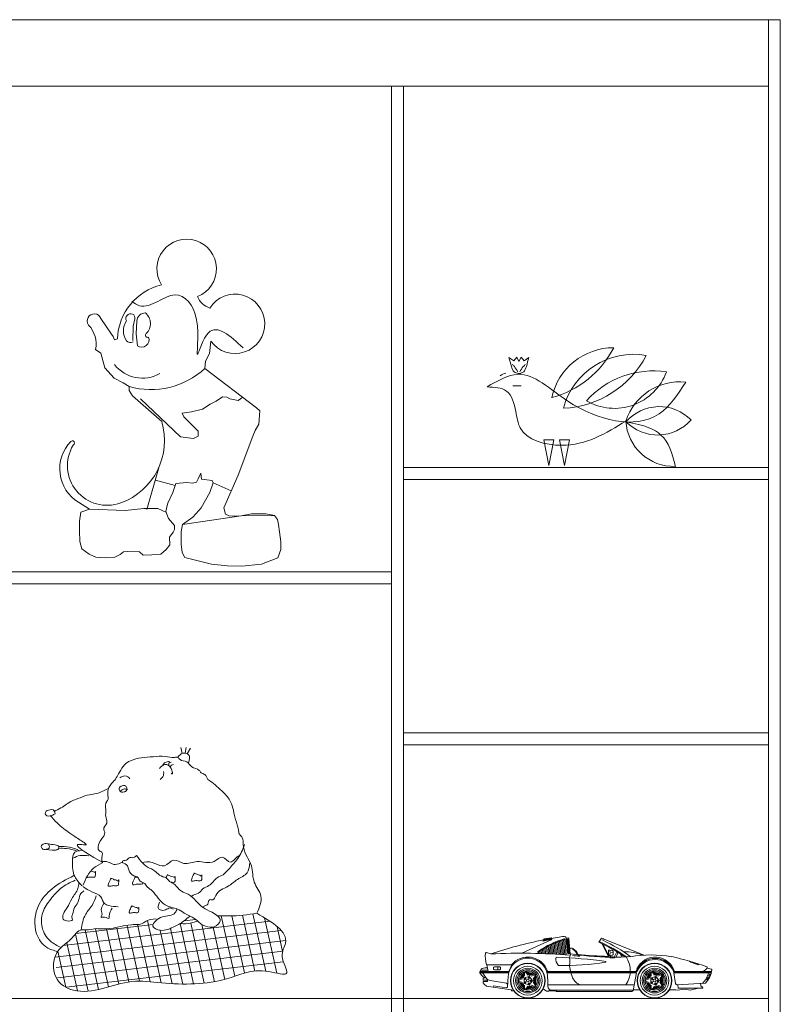
# Model space of a CAD drawing. Units: inches. Extents: x -17 to 1735, y -531 to 60.
# Tile 15 of 27: x 1734.69407 to 1734.73921, y -150.22453 to -150.16612. Entities that reach past the tile are written whole.
import ezdxf

# ---------------------------------------------------------------- set-up
doc = ezdxf.new("R2010")
doc.units = ezdxf.units.IN
doc.header["$MEASUREMENT"] = 0
doc.layers.add('A-FURN', color=242, linetype='Continuous', lineweight=18, true_color=0xcd2027)

# ---------------------------------------------------------------- blocks, each defined once
blk = doc.blocks.new('childrens_room_2')
for p, q in [((69.7359, 55.4342), (71.7959, 55.4342)), ((71.7779, 55.4342), (71.7779, 52.9342)), ((71.7959, 55.4342), (71.7959, 52.9342)), ((69.7569, 55.3342), (71.7779, 55.3342)), ((71.2099, 52.9342), (71.2099, 55.3342)), ((71.2279, 52.9342), (71.2279, 55.3342)), ((71.3868, 54.925), (71.394, 54.9202)), ((71.394, 54.9202), (71.3986, 54.9258)), ((71.3986, 54.9258), (71.4018, 54.9193)), ((71.405, 54.9258), (71.4018, 54.9193)), ((71.4096, 54.9202), (71.405, 54.9258)), ((71.4168, 54.925), (71.4096, 54.9202)), ((71.3929, 54.8824), (71.4054, 54.8824)), ((71.4392, 54.8012), (71.4468, 54.7622)), ((71.4392, 54.8012), (71.4544, 54.8012)), ((71.4544, 54.8012), (71.4468, 54.7622)), ((71.463, 54.8012), (71.4707, 54.7622)), ((71.463, 54.8012), (71.4783, 54.8012)), ((71.4783, 54.8012), (71.4707, 54.7622)), ((70.8596, 54.7608), (70.8411, 54.6961)), ((71.2279, 54.7594), (71.7779, 54.7594)), ((70.8835, 54.732), (70.8538, 54.7405)), ((71.2279, 54.7414), (71.7779, 54.7414)), ((70.9407, 54.7363), (70.9683, 54.7242)), ((70.9834, 54.6866), (70.8945, 54.6733)), ((71.0335, 54.687), (70.9834, 54.6866)), ((69.7569, 54.6022), (71.2099, 54.6022)), ((69.7569, 54.5842), (71.2099, 54.5842)), ((71.2279, 54.3594), (71.7779, 54.3594)), ((70.892, 54.3372), (70.8942, 54.3285)), ((70.9001, 54.3372), (70.8985, 54.329)), ((70.9067, 54.3366), (70.9016, 54.3281)), ((71.2279, 54.3414), (71.7779, 54.3414)), ((70.9852, 54.0846), (71.004, 54.0005)), ((71.0009, 54.0866), (71.0201, 54.0003)), ((71.0009, 54.0866), (71.0201, 54.0003)), ((70.715, 54.0389), (71.0266, 54.0757)), ((70.7341, 54.0571), (70.8504, 54.0708)), ((70.8269, 54.0706), (70.8462, 53.9844)), ((70.8417, 54.0766), (70.8627, 53.9827)), ((70.8574, 54.0788), (70.8574, 54.0787)), ((70.8911, 54.0721), (70.9114, 53.9812)), ((70.897, 54.0763), (70.9146, 54.0783)), ((70.9071, 54.0728), (70.9273, 53.9823)), ((70.9237, 54.0708), (70.943, 53.9845)), ((70.9531, 54.0837), (70.9734, 53.9928)), ((70.9693, 54.0836), (70.9884, 53.9976)), ((71.0183, 54.0809), (71.0369, 53.9974)), ((70.7027, 54.0216), (71.0435, 54.0618)), ((70.7333, 54.0562), (70.7525, 53.9702)), ((70.7481, 54.0624), (70.7681, 53.9728)), ((70.7638, 54.0643), (70.7833, 53.9768)), ((70.78, 54.064), (70.7985, 53.981)), ((70.7959, 54.0651), (70.8139, 53.9842)), ((70.8113, 54.0685), (70.8298, 53.9852)), ((70.8611, 54.0618), (70.8791, 53.9815)), ((70.8766, 54.0648), (70.8953, 53.9809)), ((70.9407, 54.0669), (70.9583, 53.9879)), ((71.0373, 54.0678), (71.0457, 54.0302)), ((70.7045, 54.006), (71.0503, 54.0468)), ((70.7201, 54.0431), (70.7363, 53.9705)), ((71.4064, 54.0275), (71.4503, 54.0477)), ((71.4398, 54.0492), (71.4379, 54.0458)), ((71.4379, 54.0458), (71.4493, 54.048)), ((71.4386, 54.046), (71.4386, 54.0467)), ((71.4391, 54.0461), (71.4391, 54.0479)), ((71.4396, 54.0462), (71.4396, 54.0489)), ((71.4512, 54.0508), (71.4398, 54.0492)), ((71.4401, 54.0463), (71.4401, 54.049)), ((71.4406, 54.0463), (71.4406, 54.049)), ((71.4411, 54.0464), (71.4411, 54.0491)), ((71.4416, 54.0465), (71.4416, 54.0492)), ((71.4422, 54.0466), (71.4422, 54.0493)), ((71.4427, 54.0467), (71.4427, 54.0494)), ((71.4432, 54.0468), (71.4432, 54.0494)), ((71.4437, 54.0468), (71.4437, 54.0495)), ((71.4442, 54.0469), (71.4442, 54.0496)), ((71.4447, 54.047), (71.4447, 54.0497)), ((71.4453, 54.0471), (71.4453, 54.0498)), ((71.4458, 54.0472), (71.4458, 54.0498)), ((71.4463, 54.0472), (71.4463, 54.0499)), ((71.4468, 54.0473), (71.4468, 54.05)), ((71.4473, 54.0474), (71.4473, 54.0501)), ((71.4478, 54.0475), (71.4478, 54.0502)), ((71.4484, 54.0476), (71.4484, 54.0503)), ((71.4489, 54.0477), (71.4489, 54.0503)), ((71.4492, 54.0398), (71.4504, 54.0263)), ((71.4493, 54.048), (71.4512, 54.0508)), ((71.4494, 54.0477), (71.4494, 54.0504)), ((71.4499, 54.0485), (71.4499, 54.0505)), ((71.4503, 54.0477), (71.4518, 54.0499)), ((71.4504, 54.0495), (71.4504, 54.0506)), ((71.4509, 54.0505), (71.4509, 54.0507)), ((71.4512, 54.0407), (71.4525, 54.0262)), ((71.4531, 54.0416), (71.4545, 54.0261)), ((71.4551, 54.0425), (71.4566, 54.0259)), ((71.4571, 54.0433), (71.4587, 54.0258)), ((71.4591, 54.0441), (71.4608, 54.0257)), ((71.4611, 54.0449), (71.4629, 54.0255)), ((71.4631, 54.0456), (71.4649, 54.0254)), ((71.4651, 54.0463), (71.467, 54.0253)), ((71.4671, 54.047), (71.4691, 54.0251)), ((71.4691, 54.0476), (71.4712, 54.0249)), ((71.4711, 54.048), (71.4732, 54.0248)), ((71.4728, 54.052), (71.475, 54.0278)), ((71.4761, 54.0506), (71.4728, 54.0503)), ((71.4773, 54.049), (71.473, 54.0487)), ((71.4742, 54.0488), (71.4762, 54.0266)), ((71.4752, 54.0489), (71.4772, 54.0267)), ((71.4762, 54.0489), (71.4782, 54.0268)), ((71.4772, 54.0496), (71.4793, 54.0263)), ((71.5263, 54.0501), (71.5223, 54.0441)), ((71.5289, 54.0496), (71.5263, 54.0501)), ((71.527, 54.0419), (71.5375, 54.0215)), ((71.5289, 54.049), (71.5283, 54.047)), ((71.5286, 54.0411), (71.5386, 54.0215)), ((71.5289, 54.049), (71.5289, 54.0496)), ((71.5908, 54.0243), (71.5289, 54.049)), ((70.7063, 53.9903), (71.0458, 54.0304)), ((70.7068, 54.0304), (70.7189, 53.9761)), ((71.3596, 54.0263), (71.353, 54.0285)), ((71.4319, 54.028), (71.4326, 54.027)), ((71.4335, 54.0308), (71.4338, 54.027)), ((71.4354, 54.0321), (71.4359, 54.027)), ((71.4374, 54.0333), (71.438, 54.0269)), ((71.4393, 54.0345), (71.44, 54.0268)), ((71.4413, 54.0356), (71.4421, 54.0267)), ((71.4433, 54.0367), (71.4442, 54.0266)), ((71.4452, 54.0378), (71.4463, 54.0265)), ((71.4472, 54.0388), (71.4483, 54.0264)), ((71.4802, 54.0259), (71.4792, 54.0243)), ((71.5367, 54.0322), (71.5367, 54.0246)), ((71.5388, 54.0322), (71.5367, 54.0322)), ((71.5383, 54.0319), (71.5395, 54.0289)), ((71.5394, 54.0277), (71.5385, 54.0241)), ((71.543, 54.0316), (71.5388, 54.0322)), ((71.5395, 54.0289), (71.5439, 54.0286)), ((71.544, 54.0303), (71.543, 54.0316)), ((71.543, 54.0244), (71.544, 54.0251)), ((71.544, 54.0251), (71.544, 54.0303)), ((71.5492, 54.0285), (71.5456, 54.0214)), ((71.551, 54.0272), (71.548, 54.0216)), ((71.5574, 54.0222), (71.555, 54.026)), ((70.7191, 53.976), (71.0467, 54.0146)), ((71.4792, 54.0243), (71.4782, 54.0203)), ((71.5367, 54.0246), (71.5374, 54.0239)), ((71.5374, 54.0239), (71.54, 54.0241)), ((71.539, 54.0204), (71.54, 54.0215)), ((71.546, 54.0204), (71.539, 54.0204)), ((71.54, 54.0241), (71.54, 54.0216)), ((71.5421, 54.0215), (71.5421, 54.0244)), ((71.5421, 54.0244), (71.543, 54.0244)), ((71.5421, 54.0215), (71.543, 54.0211)), ((71.543, 54.0211), (71.546, 54.021)), ((71.546, 54.021), (71.546, 54.0204)), ((71.6608, 54.0139), (71.659, 54.0154)), ((71.6723, 54.0098), (71.6608, 54.0139)), ((71.6705, 54.0111), (71.6633, 54.0139)), ((71.6708, 54.0114), (71.6705, 54.0111)), ((71.6732, 54.0106), (71.6723, 54.0098)), ((71.3869, 54), (71.3431, 54)), ((71.3431, 54), (71.3431, 53.998)), ((71.3869, 53.9995), (71.3431, 53.9995)), ((71.3869, 53.999), (71.3431, 53.999)), ((71.3869, 53.9985), (71.3431, 53.9985)), ((71.3864, 53.998), (71.3431, 53.998)), ((71.3455, 53.9941), (71.3431, 53.998)), ((71.3441, 54.0016), (71.3436, 54)), ((71.355, 54.0016), (71.3441, 54.0016)), ((71.3532, 53.9895), (71.3472, 53.998)), ((71.3503, 54.0052), (71.3544, 54.0052)), ((71.3529, 54.0098), (71.3911, 54.0098)), ((71.3555, 54), (71.3534, 54.0098)), ((71.3637, 54.0036), (71.3637, 54.0057)), ((71.3648, 54.0067), (71.373, 54.0067)), ((71.373, 54.0026), (71.3648, 54.0026)), ((71.3699, 54.0067), (71.3699, 54.0026)), ((71.374, 54.0057), (71.374, 54.0036)), ((71.3869, 54), (71.3911, 54.0098)), ((71.4088, 53.999), (71.4088, 53.9908)), ((71.4104, 53.9987), (71.4104, 53.9928)), ((71.4154, 53.9944), (71.4119, 53.9992)), ((71.4178, 53.9938), (71.413, 54.0003)), ((71.4256, 53.9963), (71.4178, 53.9938)), ((71.5798, 54), (71.4436, 54)), ((71.5788, 53.9995), (71.4438, 53.9995)), ((71.5787, 53.999), (71.4439, 53.999)), ((71.5785, 53.9985), (71.4441, 53.9985)), ((71.579, 53.998), (71.4442, 53.998)), ((71.4778, 54.0094), (71.4779, 54.0079)), ((71.4779, 54.0079), (71.4798, 54.0001)), ((71.482, 53.9924), (71.4803, 53.998)), ((71.5798, 54), (71.5494, 54)), ((71.5789, 53.998), (71.5741, 53.9713)), ((71.5789, 54), (71.5784, 53.998)), ((71.5997, 53.999), (71.5997, 53.9908)), ((71.6013, 53.9987), (71.6013, 53.9928)), ((71.6064, 53.9944), (71.6029, 53.9992)), ((71.6088, 53.9938), (71.604, 54.0003)), ((71.6165, 53.9963), (71.6088, 53.9938)), ((71.6924, 54), (71.6348, 54)), ((71.6924, 53.9995), (71.6348, 53.9995)), ((71.6922, 53.999), (71.6348, 53.999)), ((71.6921, 53.9985), (71.6348, 53.9985)), ((71.6356, 54), (71.6362, 53.998)), ((71.6919, 53.998), (71.6356, 53.998)), ((71.6356, 53.998), (71.638, 53.9817)), ((71.6795, 54.0005), (71.6708, 54)), ((71.6919, 54.0035), (71.6852, 54.0047)), ((71.6894, 53.9959), (71.6883, 53.9933)), ((71.6909, 53.9959), (71.6894, 53.9959)), ((71.3482, 53.9896), (71.3482, 53.9866)), ((71.3482, 53.9866), (71.3544, 53.9866)), ((71.3482, 53.985), (71.3482, 53.983)), ((71.3544, 53.985), (71.3482, 53.985)), ((71.3482, 53.983), (71.3493, 53.9809)), ((71.3493, 53.9809), (71.3529, 53.9778)), ((71.3544, 53.9866), (71.3544, 53.985)), ((71.3833, 53.9825), (71.3583, 53.9861)), ((71.3844, 53.9809), (71.3833, 53.9825)), ((71.3844, 53.9763), (71.3855, 53.9926)), ((71.4088, 53.9908), (71.4011, 53.9883)), ((71.4011, 53.9839), (71.4088, 53.9813)), ((71.4074, 53.9887), (71.4018, 53.9869)), ((71.4018, 53.9853), (71.4074, 53.9834)), ((71.4088, 53.9813), (71.4088, 53.9732)), ((71.4098, 53.9893), (71.4098, 53.9828)), ((71.4167, 53.9923), (71.4105, 53.9903)), ((71.4105, 53.9819), (71.4167, 53.9799)), ((71.4217, 53.9867), (71.4179, 53.9919)), ((71.4179, 53.9802), (71.4217, 53.9855)), ((71.4258, 53.9947), (71.4202, 53.9929)), ((71.4233, 53.9886), (71.4268, 53.9934)), ((71.4268, 53.9788), (71.4233, 53.9836)), ((71.4234, 53.9861), (71.4282, 53.9927)), ((71.4282, 53.9795), (71.4234, 53.9861)), ((71.4452, 53.9889), (71.4456, 53.9776)), ((71.5997, 53.9908), (71.592, 53.9883)), ((71.592, 53.9839), (71.5997, 53.9813)), ((71.5984, 53.9887), (71.5927, 53.9869)), ((71.5927, 53.9853), (71.5984, 53.9834)), ((71.5997, 53.9813), (71.5997, 53.9732)), ((71.6008, 53.9893), (71.6008, 53.9828)), ((71.6077, 53.9923), (71.6015, 53.9903)), ((71.6015, 53.9819), (71.6077, 53.9799)), ((71.6126, 53.9867), (71.6088, 53.9919)), ((71.6088, 53.9802), (71.6126, 53.9855)), ((71.6168, 53.9947), (71.6111, 53.9929)), ((71.6142, 53.9886), (71.6177, 53.9934)), ((71.6177, 53.9788), (71.6142, 53.9836)), ((71.6143, 53.9861), (71.6191, 53.9927)), ((71.6191, 53.9795), (71.6143, 53.9861)), ((71.6825, 53.9822), (71.6402, 53.9799)), ((71.6764, 53.9768), (71.6754, 53.982)), ((71.6873, 53.9912), (71.6847, 53.9871)), ((71.6847, 53.9871), (71.6868, 53.9871)), ((71.6888, 53.9912), (71.6873, 53.9912)), ((71.6883, 53.9933), (71.6904, 53.9933)), ((71.3529, 53.9778), (71.3632, 53.9761)), ((71.3632, 53.9761), (71.3637, 53.9781)), ((71.39, 53.9721), (71.3632, 53.9761)), ((71.3833, 53.9752), (71.3637, 53.9781)), ((71.3833, 53.9752), (71.3844, 53.9763)), ((71.3911, 53.9706), (71.39, 53.9721)), ((71.3926, 53.9706), (71.3911, 53.9706)), ((71.3937, 53.9716), (71.3926, 53.9706)), ((71.4104, 53.9794), (71.4104, 53.9734)), ((71.4119, 53.9729), (71.4154, 53.9777)), ((71.413, 53.9718), (71.4178, 53.9784)), ((71.4178, 53.9784), (71.4256, 53.9759)), ((71.4202, 53.9793), (71.4258, 53.9774)), ((71.4401, 53.9727), (71.438, 53.9732)), ((71.4432, 53.9701), (71.4401, 53.9727)), ((71.4463, 53.9701), (71.4432, 53.9701)), ((71.4455, 53.9799), (71.5756, 53.9799)), ((71.4484, 53.9716), (71.4463, 53.9701)), ((71.4571, 53.9706), (71.4473, 53.9706)), ((71.4515, 53.9716), (71.4484, 53.9716)), ((71.4518, 53.9716), (71.5738, 53.9716)), ((71.4587, 53.9696), (71.4561, 53.9716)), ((71.4587, 53.9696), (71.572, 53.9696)), ((71.5748, 53.9721), (71.5846, 53.9721)), ((71.6013, 53.9794), (71.6013, 53.9734)), ((71.6029, 53.9729), (71.6064, 53.9777)), ((71.604, 53.9718), (71.6088, 53.9784)), ((71.6088, 53.9784), (71.6165, 53.9759)), ((71.6111, 53.9793), (71.6168, 53.9774)), ((71.6285, 53.9721), (71.6383, 53.9721)), ((71.6383, 53.9721), (71.6403, 53.9716)), ((71.6403, 53.9716), (71.6527, 53.9732)), ((71.6419, 53.9747), (71.6414, 53.9799)), ((71.679, 53.9747), (71.6419, 53.9747)), ((71.6527, 53.9732), (71.6599, 53.9716)), ((71.6599, 53.9716), (71.6728, 53.9747)), ((71.6788, 53.9768), (71.6764, 53.9768)), ((71.6788, 53.9768), (71.679, 53.9758)), ((71.679, 53.9758), (71.679, 53.9747)), ((69.7569, 53.9594), (71.7779, 53.9594))]:
    blk.add_line(p, q)
for points in [[(70.8631, 55.0345, -2.780632), (70.9175, 55.0169, 0.231731), (70.9359, 54.9997, -3.269279), (70.9375, 54.9496), (70.9352, 54.9314), (70.9293, 54.9197), (70.9285, 54.9087), (71.0064, 54.8493), (71.0111, 54.8446), (71.0099, 54.8246), (71.0041, 54.8149), (71.0005, 54.8066), (70.9787, 54.748), (70.9571, 54.6987), (70.9595, 54.6889), (70.9653, 54.6866), (70.9724, 54.6858), (70.9834, 54.6866), (70.9986, 54.6897), (71.0205, 54.6893), (71.0335, 54.687), (71.0378, 54.6811), (71.0393, 54.6733), (71.0409, 54.6624), (71.0428, 54.6471), (71.0428, 54.6358), (71.0385, 54.6232), (71.0139, 54.6139), (70.9841, 54.6107), (70.9626, 54.6111), (70.9383, 54.6135), (70.9121, 54.6201), (70.8984, 54.6236), (70.8941, 54.6315), (70.8929, 54.644), (70.8929, 54.6624), (70.8945, 54.6733), (70.9102, 54.6846), (70.9192, 54.6948), (70.9227, 54.6987), (70.936, 54.7218), (70.9407, 54.7363), (70.9395, 54.7398), (70.9235, 54.7417), (70.9223, 54.7507), (70.9184, 54.7421), (70.9156, 54.7371), (70.9098, 54.7359), (70.9012, 54.7367), (70.8847, 54.7351), (70.8835, 54.732), (70.88, 54.7218), (70.8726, 54.7058), (70.8718, 54.7022), (70.8698, 54.6929), (70.8734, 54.6823), (70.8824, 54.6721), (70.8828, 54.6659), (70.8804, 54.662), (70.8753, 54.6545), (70.8757, 54.6428), (70.8702, 54.6358), (70.8618, 54.6286), (70.8485, 54.6278), (70.8356, 54.6271), (70.8301, 54.6325), (70.8117, 54.6329), (70.8058, 54.6325), (70.8007, 54.6282), (70.7925, 54.6243), (70.7792, 54.6231), (70.7639, 54.6243), (70.7542, 54.629), (70.7432, 54.6368), (70.7397, 54.6478), (70.7393, 54.6638), (70.7393, 54.6783), (70.7416, 54.692), (70.7546, 54.6967), (70.7377, 54.707, -0.480393), (70.7264, 54.7986, -1.257082), (70.7299, 54.7931, 0.706408), (70.8015, 54.7059, 0.397958), (70.8634, 54.8287), (70.8191, 54.8672), (70.8144, 54.8754), (70.8141, 54.8813), (70.8054, 54.8868), (70.7917, 54.8938), (70.7777, 54.9095), (70.7714, 54.9318), (70.7637, 54.9371)], [(70.7879, 54.9602), (70.7903, 54.9569), (70.7923, 54.9515), (70.7966, 54.9534, -0.337972), (70.8631, 55.0345)], [(70.7879, 54.9602), (70.7715, 54.984, 1.147535), (70.7531, 54.9741, -0.239038), (70.7637, 54.9371, 0.932314)], [(70.8197, 54.9508), (70.8204, 54.9721), (70.823, 54.9833, 0.357136), (70.8193, 54.9904, 0.713549), (70.8101, 54.9802, 0.314811), (70.8105, 54.9504, 0.383013), (70.8201, 54.9485, -0.242652)], [(70.8268, 54.9428), (70.8251, 54.9607), (70.826, 54.98, -0.410066), (70.8388, 54.9922, -0.451179), (70.84, 54.9611, 0.84041), (70.8437, 54.9557, -0.740597), (70.8268, 54.9428)]]:
    blk.add_lwpolyline(points, format="xyb")
for points in [[(70.8312, 54.8628), (70.8916, 54.8057), (70.9111, 54.8031), (70.9182, 54.8064), (70.9182, 54.8142), (70.8968, 54.8356), (70.8942, 54.8414), (70.9085, 54.8433), (70.9247, 54.8472), (70.9364, 54.855), (70.9454, 54.8595), (70.9552, 54.866), (70.9617, 54.8654), (70.9662, 54.8628), (70.9785, 54.8602), (70.9857, 54.8654)], [(70.7546, 54.6967), (70.8085, 54.6945), (70.8362, 54.6978), (70.8574, 54.6978), (70.8704, 54.6913)]]:
    blk.add_lwpolyline(points)
for centre, radius in [((71.4153, 53.9861), 0.0263), ((71.4153, 53.9861), 0.0258), ((71.6063, 53.9861), 0.0263), ((71.6063, 53.9861), 0.0258), ((71.4153, 53.9861), 0.0217), ((71.4153, 53.9861), 0.0186), ((71.4153, 53.9861), 0.0165), ((71.4153, 53.9861), 0.0144), ((71.6063, 53.9861), 0.0217), ((71.6063, 53.9861), 0.0186), ((71.6063, 53.9861), 0.0165), ((71.6063, 53.9861), 0.0144), ((71.4115, 53.9889), 0.00103), ((71.4115, 53.9833), 0.00103), ((71.4153, 53.9861), 0.00206), ((71.4168, 53.9816), 0.00103), ((71.4168, 53.9905), 0.00103), ((71.42, 53.986), 0.00103), ((71.6024, 53.9833), 0.00103), ((71.6025, 53.9889), 0.00103), ((71.6063, 53.9861), 0.00206), ((71.6078, 53.9905), 0.00103), ((71.6077, 53.9816), 0.00103), ((71.611, 53.986), 0.00103)]:
    blk.add_circle(centre, radius)
for centre, radius, start, end in [((71.5443, 54.8449), 0.0949, 89.6755, 168.0465), ((71.4129, 55.008), 0.1485, 285.0539, 332.6681), ((71.5747, 54.8206), 0.1093, 79.8911, 165.1278), ((71.4622, 54.9972), 0.1487, 272.6693, 332.3497), ((70.8341, 54.9473), 0.0533, 218.1081, 299.9312), ((70.8468, 54.9973), 0.1205, 254.2406, 312.7067), ((71.3844, 54.8856), 0.016, 97.5951, 131.4079), ((71.6043, 54.7699), 0.135, 81.5012, 138.2063), ((71.5458, 54.9319), 0.0834, 239.6168, 340.0908), ((71.6448, 54.8026), 0.086, 84.3179, 161.874), ((71.6137, 54.7841), 0.067, 44.6425, 138.8712), ((71.6354, 54.8335), 0.0725, 183.2503, 272.0156), ((71.6109, 54.8753), 0.067, 224.6425, 318.8712), ((70.8072, 54.2845), 0.01, 36.043, 134.9152), ((71.5596, 53.4338), 0.6254, 101.1376, 108.6505), ((71.5096, 53.9155), 0.1392, 106.6287, 124.2618), ((71.5096, 53.9155), 0.1382, 106.6287, 124.2618), ((71.5596, 53.4338), 0.6254, 98.9092, 100.0579), ((71.4696, 54.0223), 0.0301, 83.9156, 103.1755), ((71.4701, 54.0479), 0.00103, 5.1944, 106.6287), ((71.4762, 54.0495), 0.00103, 5.1944, 94.1185), ((71.4049, 53.7876), 0.282, 56.1253, 65.4116), ((71.4049, 53.7876), 0.2831, 55.8423, 65.3782), ((71.4049, 53.7876), 0.2872, 54.7598, 64.5537), ((71.3955, 54.0217), 0.0443, 172.226, 195.5692), ((71.3527, 54.0275), 0.00103, 71.5651, 172.226), ((71.4047, 53.1697), 0.8578, 85.0164, 93.0145), ((71.4324, 54.0289), 0.00206, 124.2618, 239.656), ((71.4324, 54.0289), 0.00103, 124.2618, 239.656), ((71.4761, 54.0279), 0.00103, 185.1944, 260.9327), ((71.5443, 54.4557), 0.4342, 260.9327, 269.4307), ((71.4805, 54.0303), 0.00483, 56.9829, 113.5542), ((71.4758, 54.0204), 0.0147, 17.6367, 62.3192), ((71.4758, 54.0204), 0.0157, 16.3877, 62.3192), ((71.5443, 54.4557), 0.4332, 262.8735, 269.0206), ((71.5501, 54.0278), 0.00106, 324.9605, 141.986), ((71.5622, 53.9566), 0.0729, 68.2312, 91.8676), ((71.6011, 53.8419), 0.1829, 80.256, 99.744), ((71.4153, 53.9902), 0.0299, 357.5047, 175.4783), ((71.4153, 53.9902), 0.0315, 18.1482, 141.4681), ((71.4586, 54.0201), 0.00103, 88.8129, 175.6099), ((71.4732, 54.019), 0.0157, 175.6099, 218.626), ((71.4318, 53.2474), 0.7743, 82.5112, 88.0167), ((71.4653, 54.4476), 0.4389, 269.54, 278.8423), ((71.4607, 54.0155), 0.0181, 340.4628, 15.1938), ((71.4047, 53.1697), 0.8578, 84.0569, 84.7873), ((71.5326, 54.0145), 0.000516, 279.6646, 83.3016), ((71.5443, 54.4557), 0.4342, 269.7012, 273.4064), ((71.5323, 54.0011), 0.0375, 325.6886, 33.9543), ((71.6073, 53.9881), 0.0315, 22.151, 156.6372), ((71.6073, 53.9918), 0.0299, 16.0134, 156.6372), ((71.6073, 53.9881), 0.0299, 23.3628, 156.6372), ((71.5236, 53.5467), 0.4878, 70.6707, 77.1477), ((71.3496, 53.9993), 0.00591, 82.9525, 157.5604), ((71.3648, 54.0057), 0.00103, 90, 180), ((71.3648, 54.0036), 0.00103, 180, 270), ((71.373, 54.0057), 0.00103, 0, 90), ((71.373, 54.0036), 0.00103, 270, 0), ((71.4153, 53.9861), 0.0123, 122.0923, 165.9077), ((71.4153, 53.9861), 0.0112, 125.6367, 162.3633), ((71.4153, 53.9861), 0.0134, 106.5619, 109.4381), ((71.4153, 53.9861), 0.0123, 50.0923, 93.9077), ((71.4153, 53.9861), 0.0112, 53.6367, 90.3633), ((71.4153, 53.9861), 0.0102, 57.6558, 86.3442), ((71.4153, 53.9861), 0.0092, 63.2165, 80.7835), ((71.4617, 54.0098), 0.00103, 218.626, 270.3731), ((71.6063, 53.9861), 0.0123, 122.0923, 165.9077), ((71.6063, 53.9861), 0.0112, 125.6367, 162.3633), ((71.6063, 53.9861), 0.0134, 106.5619, 109.4381), ((71.6063, 53.9861), 0.0123, 50.0923, 93.9077), ((71.6063, 53.9861), 0.0112, 53.6367, 90.3633), ((71.6063, 53.9861), 0.0102, 57.6558, 86.3442), ((71.6063, 53.9861), 0.0092, 63.2165, 80.7835), ((71.6548, 54.0064), 0.034, 314.0815, 345.6357), ((71.6786, 54.008), 0.00751, 277.3344, 341.6585), ((71.659, 54.0064), 0.034, 315.3221, 353.2753), ((71.6847, 54.0059), 0.00103, 341.6585, 73.9092), ((71.6917, 54.0025), 0.00103, 353.2753, 80.5377), ((71.3522, 53.9989), 0.00826, 215.2176, 271.2671), ((71.3522, 53.9824), 0.00826, 88.7329, 118.6877), ((71.3599, 53.9942), 0.00826, 215.2176, 258.6901), ((71.4153, 53.9861), 0.0134, 178.5619, 181.4381), ((71.4153, 53.9861), 0.0123, 194.0923, 237.9077), ((71.4153, 53.9861), 0.0112, 197.6367, 234.3633), ((71.4153, 53.9861), 0.0102, 129.6558, 158.3442), ((71.4153, 53.9861), 0.0102, 201.6558, 230.3442), ((71.4153, 53.9861), 0.0092, 135.2165, 152.7835), ((71.4153, 53.9861), 0.0092, 207.2165, 224.7835), ((71.4109, 53.9893), 0.00103, 108, 180), ((71.4109, 53.9828), 0.00103, 180, 252), ((71.417, 53.9913), 0.00103, 36, 108), ((71.4209, 53.9861), 0.00103, 324, 36), ((71.4153, 53.9861), 0.0092, 351.2165, 8.7835), ((71.4153, 53.9861), 0.0102, 345.6558, 14.3442), ((71.4153, 53.9861), 0.0134, 34.5619, 37.4381), ((71.4153, 53.9861), 0.0112, 341.6367, 18.3633), ((71.4153, 53.9861), 0.0123, 338.0923, 21.9077), ((71.5023, 53.9991), 0.0213, 198.287, 243.6279), ((71.6063, 53.9861), 0.0134, 178.5619, 181.4381), ((71.6063, 53.9861), 0.0123, 194.0923, 237.9077), ((71.6063, 53.9861), 0.0112, 197.6367, 234.3633), ((71.6063, 53.9861), 0.0102, 129.6558, 158.3442), ((71.6063, 53.9861), 0.0102, 201.6558, 230.3442), ((71.6063, 53.9861), 0.0092, 135.2165, 152.7835), ((71.6063, 53.9861), 0.0092, 207.2165, 224.7835), ((71.6018, 53.9893), 0.00103, 108, 180), ((71.6018, 53.9828), 0.00103, 180, 252), ((71.608, 53.9913), 0.00103, 36, 108), ((71.6118, 53.9861), 0.00103, 324, 36), ((71.6063, 53.9861), 0.0092, 351.2165, 8.7835), ((71.6063, 53.9861), 0.0102, 345.6558, 14.3442), ((71.6063, 53.9861), 0.0134, 34.5619, 37.4381), ((71.6063, 53.9861), 0.0112, 341.6367, 18.3633), ((71.6063, 53.9861), 0.0123, 338.0923, 21.9077), ((71.64, 53.982), 0.00206, 188.4513, 273.0713), ((71.6824, 53.9832), 0.00103, 273.0713, 315.3221), ((71.4153, 53.9861), 0.0134, 250.5619, 253.4381), ((71.4153, 53.9861), 0.0123, 266.0923, 309.9077), ((71.4153, 53.9861), 0.0112, 269.6367, 306.3633), ((71.4153, 53.9861), 0.0102, 273.6558, 302.3442), ((71.417, 53.9808), 0.00103, 252, 324), ((71.4153, 53.9861), 0.0092, 279.2165, 296.7835), ((71.4153, 53.9861), 0.0134, 322.5619, 325.4381), ((71.4518, 53.9778), 0.00619, 181.9827, 270), ((71.572, 53.9716), 0.00206, 270, 349.6952), ((71.6063, 53.9861), 0.0134, 250.5619, 253.4381), ((71.6063, 53.9861), 0.0123, 266.0923, 309.9077), ((71.6063, 53.9861), 0.0112, 269.6367, 306.3633), ((71.6063, 53.9861), 0.0102, 273.6558, 302.3442), ((71.608, 53.9808), 0.00103, 252, 324), ((71.6063, 53.9861), 0.0092, 279.2165, 296.7835), ((71.6063, 53.9861), 0.0134, 322.5619, 325.4381)]:
    blk.add_arc(centre, radius, start, end)
for points, knots in [([(70.8184, 55.0097), (70.8221, 55.007), (70.8338, 54.9986), (70.8577, 55.0092), (70.8906, 55.0282), (70.9259, 54.9891), (70.911, 54.9029), (70.9347, 54.9871), (70.9666, 54.9577), (70.986, 54.9398)], [0, 0, 0, 0, 0.0131197, 0.0415435, 0.0693534, 0.1189401, 0.1710087, 0.2073805, 0.2642233, 0.2642233, 0.2642233, 0.2642233]), ([(71.3868, 54.925), (71.388, 54.9206), (71.39, 54.9135), (71.3933, 54.9028), (71.399, 54.9014), (71.4016, 54.9008)], [0, 0, 0, 0, 0.01394418, 0.02289953, 0.0304523, 0.0304523, 0.0304523, 0.0304523]), ([(71.4168, 54.925), (71.4156, 54.9206), (71.4137, 54.9135), (71.4103, 54.9026), (71.4044, 54.9014), (71.4016, 54.9008)], [0, 0, 0, 0, 0.01394418, 0.02289953, 0.03082583, 0.03082583, 0.03082583, 0.03082583]), ([(71.3538, 54.8808), (71.3696, 54.89), (71.4123, 54.9149), (71.4849, 54.8387), (71.603, 54.8097), (71.6414, 54.8696), (71.6534, 54.8882)], [0, 0, 0, 0, 0.050303, 0.135778, 0.2748013, 0.3373841, 0.3373841, 0.3373841, 0.3373841]), ([(71.3918, 54.9148), (71.3929, 54.9137), (71.3963, 54.9105), (71.3986, 54.9064), (71.4002, 54.9036)], [0, 0, 0, 0, 0.00453223, 0.01408632, 0.01408632, 0.01408632, 0.01408632]), ([(71.4117, 54.9146), (71.4106, 54.9136), (71.4071, 54.9104), (71.4047, 54.9063), (71.4031, 54.9035)], [0, 0, 0, 0, 0.00453223, 0.01408632, 0.01408632, 0.01408632, 0.01408632]), ([(71.3538, 54.8808), (71.3649, 54.8804), (71.3884, 54.8797), (71.3972, 54.8461), (71.4033, 54.8035), (71.4842, 54.7808), (71.5334, 54.8111), (71.5631, 54.8294)], [0, 0, 0, 0, 0.029981, 0.0638233, 0.0892818, 0.1569362, 0.2606419, 0.2606419, 0.2606419, 0.2606419]), ([(71.5632, 54.8282), (71.5919, 54.8232), (71.6246, 54.8094), (71.6326, 54.7818), (71.638, 54.7611)], [3447.290732, 3447.290732, 3447.290732, 3447.290732, 4243.521396, 5244.846704, 5244.846704, 5244.846704, 5244.846704]), ([(70.8503, 54.3234), (70.8386, 54.3228), (70.8232, 54.322), (70.8059, 54.3116), (70.8019, 54.3032), (70.797, 54.2961), (70.7947, 54.29), (70.7887, 54.2846), (70.7843, 54.279), (70.7823, 54.273), (70.7814, 54.266), (70.7844, 54.2593), (70.7775, 54.254), (70.7792, 54.2459), (70.7789, 54.2386), (70.7787, 54.2334), (70.7808, 54.2287), (70.7814, 54.2215), (70.7739, 54.2161), (70.7799, 54.2067), (70.7696, 54.1985), (70.7647, 54.1824), (70.7767, 54.1792), (70.7714, 54.1704), (70.7735, 54.1659), (70.774, 54.165)], [0, 0, 0, 0, 219.159921, 287.663278, 372.750424, 390.389024, 451.893717, 493.538516, 541.005164, 587.230906, 611.729041, 678.188313, 691.620931, 768.166453, 806.143293, 836.602939, 864.377233, 902.354072, 966.053688, 996.0796, 1081.012481, 1185.879975, 1207.123995, 1283.077449, 1302.366322, 1302.366322, 1302.366322, 1302.366322]), ([(70.8503, 54.3234), (70.8565, 54.3241), (70.8675, 54.3253), (70.8793, 54.3214), (70.888, 54.3235), (70.8917, 54.3164), (70.9026, 54.3183), (70.9076, 54.3057), (70.9192, 54.3061), (70.9225, 54.2982), (70.9302, 54.2976), (70.9314, 54.29), (70.9425, 54.2828), (70.9544, 54.2722), (70.9677, 54.2575), (70.971, 54.2453), (70.9731, 54.2334), (70.9766, 54.2237), (70.9793, 54.214), (70.9793, 54.2071), (70.9874, 54.2011), (70.984, 54.1811), (71.0019, 54.162), (70.9993, 54.1341), (71.018, 54.1131), (71.0108, 54.0964), (71.0069, 54.0875)], [0, 0, 0, 0, 0.0184035, 0.0325789, 0.0373025, 0.0420369, 0.0527164, 0.0634089, 0.0760054, 0.0805621, 0.0867538, 0.0953843, 0.0991638, 0.1260367, 0.143618, 0.1572394, 0.1632561, 0.1798707, 0.1877421, 0.1937588, 0.1991999, 0.2154002, 0.246082, 0.2710254, 0.2942493, 0.3208889, 0.3208889, 0.3208889, 0.3208889]), ([(70.8879, 54.323), (70.8899, 54.3255), (70.8942, 54.3307), (70.9053, 54.3278), (70.9055, 54.3198), (70.9043, 54.3161), (70.9036, 54.314)], [0, 0, 0, 0, 0.0091093, 0.01924587, 0.02441068, 0.03102537, 0.03102537, 0.03102537, 0.03102537]), ([(70.86, 54.306), (70.8623, 54.3084), (70.8667, 54.3128), (70.8769, 54.3111), (70.8819, 54.2952), (70.8779, 54.2981), (70.8775, 54.2985)], [0, 0, 0, 0, 0.00939944, 0.0173366, 0.02942409, 0.03086013, 0.03086013, 0.03086013, 0.03086013]), ([(70.8651, 54.3112), (70.8662, 54.3126), (70.8688, 54.3157), (70.8728, 54.3161), (70.8751, 54.3164)], [0, 0, 0, 0, 0.00506849, 0.01163851, 0.01163851, 0.01163851, 0.01163851]), ([(70.8739, 54.3112), (70.8739, 54.3121), (70.874, 54.3143), (70.8762, 54.3148), (70.8775, 54.3152)], [0, 0, 0, 0, 0.002421308, 0.005983967, 0.005983967, 0.005983967, 0.005983967]), ([(70.8767, 54.3084), (70.8771, 54.3093), (70.878, 54.3112), (70.8801, 54.3115), (70.8811, 54.3116)], [0, 0, 0, 0, 0.002871137, 0.005771228, 0.005771228, 0.005771228, 0.005771228]), ([(70.8663, 54.3012), (70.8664, 54.2983), (70.8665, 54.2933), (70.8625, 54.2905), (70.8608, 54.2893)], [0, 0, 0, 0, 0.00805023, 0.01397039, 0.01397039, 0.01397039, 0.01397039]), ([(70.8107, 54.2768), (70.81, 54.2781), (70.8084, 54.2806), (70.8039, 54.2802), (70.801, 54.2785), (70.7989, 54.2759), (70.7997, 54.2726), (70.8024, 54.2696), (70.8069, 54.2703), (70.8103, 54.2717), (70.8113, 54.2746), (70.8109, 54.276), (70.8107, 54.2768)], [0, 0, 0, 0, 0.00405876, 0.00822906, 0.01159062, 0.01459614, 0.01713079, 0.02125745, 0.02535249, 0.02984432, 0.03148227, 0.03400113, 0.03400113, 0.03400113, 0.03400113]), ([(70.7011, 54.2411), (70.7046, 54.2427), (70.7142, 54.2471), (70.7248, 54.2561), (70.7387, 54.2609), (70.7506, 54.2662), (70.7672, 54.2674), (70.7773, 54.2728), (70.783, 54.2758)], [0, 0, 0, 0, 0.0116539, 0.03159237, 0.04066447, 0.0555855, 0.07045457, 0.08961689, 0.08961689, 0.08961689, 0.08961689]), ([(70.8106, 54.2735), (70.81, 54.2742), (70.8086, 54.2756), (70.8052, 54.2746), (70.8026, 54.2732), (70.8017, 54.2715), (70.8015, 54.2709)], [0, 0, 0, 0, 0.00271634, 0.00557539, 0.00949311, 0.01130026, 0.01130026, 0.01130026, 0.01130026]), ([(70.703, 54.2374), (70.7023, 54.24), (70.7011, 54.2444), (70.6939, 54.2434), (70.6871, 54.2418), (70.6883, 54.233), (70.6971, 54.2346), (70.7013, 54.2366), (70.703, 54.2374)], [0, 0, 0, 0, 0.00698779, 0.01148071, 0.01977129, 0.02373924, 0.03274257, 0.03875645, 0.03875645, 0.03875645, 0.03875645]), ([(70.6951, 54.2351), (70.6985, 54.2313), (70.7073, 54.2214), (70.7237, 54.2089), (70.7353, 54.2012), (70.7554, 54.1888), (70.7208, 54.1953), (70.7501, 54.1782), (70.7745, 54.1639)], [0, 0, 0, 0, 0.0154163, 0.0403412, 0.0565833, 0.0702455, 0.0787996, 0.1223226, 0.1223226, 0.1223226, 0.1223226]), ([(70.6927, 54.192), (70.6905, 54.1925), (70.6864, 54.1935), (70.6805, 54.1889), (70.6835, 54.184), (70.6877, 54.1837), (70.6904, 54.1848), (70.6933, 54.1848), (70.6946, 54.1881), (70.6935, 54.1903), (70.6927, 54.192)], [0, 0, 0, 0, 0.00655182, 0.01252414, 0.01677918, 0.01999142, 0.02432705, 0.02590444, 0.02784131, 0.03323975, 0.03323975, 0.03323975, 0.03323975]), ([(70.6927, 54.192), (70.6958, 54.1916), (70.7007, 54.191), (70.7088, 54.1896), (70.7082, 54.1835), (70.6977, 54.1819), (70.6902, 54.1833), (70.6843, 54.1843)], [0, 0, 0, 0, 0.00999672, 0.0161539, 0.01941415, 0.02458379, 0.04334789, 0.04334789, 0.04334789, 0.04334789]), ([(70.7394, 54.1819), (70.7345, 54.1842), (70.7245, 54.1884), (70.7137, 54.1883), (70.7081, 54.1881)], [21.853899, 21.853899, 21.853899, 21.853899, 99.616764, 179.646874, 179.646874, 179.646874, 179.646874]), ([(70.9883, 54.1911), (70.9854, 54.1837), (70.9802, 54.1704), (70.9667, 54.1573), (70.9578, 54.1455), (70.9441, 54.1411), (70.9375, 54.129), (70.9249, 54.1258), (70.9196, 54.1161), (70.9103, 54.1163), (70.9085, 54.113), (70.9083, 54.1127)], [0, 0, 0, 0, 148.663269, 267.623843, 357.982231, 421.109249, 530.360405, 597.090395, 653.533218, 724.476551, 730.449387, 730.449387, 730.449387, 730.449387]), ([(70.7355, 54.1812), (70.7304, 54.183), (70.7214, 54.1857), (70.7121, 54.1856), (70.7081, 54.1854)], [12.053059, 12.053059, 12.053059, 12.053059, 90.710426, 148.332878, 148.332878, 148.332878, 148.332878]), ([(70.7425, 54.1822), (70.7386, 54.1819), (70.7293, 54.181), (70.7284, 54.1617), (70.7292, 54.1436), (70.739, 54.1335), (70.7432, 54.1291)], [0, 0, 0, 0, 0.01070517, 0.0249108, 0.04790907, 0.06556289, 0.06556289, 0.06556289, 0.06556289]), ([(70.7536, 54.1739), (70.7491, 54.1746), (70.7407, 54.1759), (70.7331, 54.1722), (70.7294, 54.1705)], [0, 0, 0, 0, 0.01312084, 0.02490384, 0.02490384, 0.02490384, 0.02490384]), ([(70.8255, 54.1744), (70.8314, 54.1664), (70.8381, 54.1575), (70.851, 54.1534), (70.8563, 54.1478), (70.863, 54.1428), (70.8711, 54.1413), (70.8743, 54.1354), (70.8842, 54.1317), (70.8902, 54.1205), (70.91, 54.1151), (70.9209, 54.0966), (70.9393, 54.09), (70.9572, 54.0779), (70.9424, 54.0649), (70.9318, 54.0672), (70.921, 54.0714), (70.9135, 54.0811), (70.8998, 54.0853), (70.8884, 54.0954), (70.8669, 54.0969), (70.8562, 54.1134), (70.8473, 54.1235), (70.8413, 54.1264), (70.8386, 54.1337), (70.83, 54.1346), (70.8282, 54.1426), (70.8192, 54.1438), (70.8137, 54.1509), (70.8124, 54.1607), (70.8069, 54.1628), (70.8035, 54.1641)], [0, 0, 0, 0, 0.0283579, 0.0318404, 0.0401203, 0.0508818, 0.0564072, 0.0637213, 0.0689346, 0.0872436, 0.0979478, 0.1281756, 0.1435053, 0.161339, 0.1740235, 0.1870542, 0.1925586, 0.208601, 0.2217304, 0.2343239, 0.2531471, 0.2816435, 0.2880435, 0.2936055, 0.3009758, 0.3090781, 0.315176, 0.3215449, 0.3334648, 0.3395958, 0.3494659, 0.3494659, 0.3494659, 0.3494659]), ([(70.8255, 54.1744), (70.8234, 54.1728), (70.82, 54.1702), (70.8138, 54.1726), (70.8122, 54.1681), (70.8085, 54.1673), (70.8041, 54.1672), (70.8044, 54.1648), (70.8045, 54.1642)], [0, 0, 0, 0, 0.0074172, 0.01203141, 0.01589691, 0.01854965, 0.02345898, 0.02513548, 0.02513548, 0.02513548, 0.02513548]), ([(70.9811, 54.1749), (70.9809, 54.1748), (70.9756, 54.1734), (70.968, 54.1573), (70.9549, 54.1776), (70.9393, 54.159), (70.9183, 54.1698), (70.8982, 54.1585), (70.8808, 54.1726), (70.8685, 54.1549), (70.8526, 54.164), (70.8411, 54.1664), (70.835, 54.1641), (70.8341, 54.1637)], [66.486016, 66.486016, 66.486016, 66.486016, 71.409099, 178.76834, 266.874671, 357.227055, 518.881407, 647.068977, 749.366568, 850.336891, 945.548877, 1050.108048, 1067.875676, 1067.875676, 1067.875676, 1067.875676]), ([(70.7745, 54.1639), (70.7698, 54.1615), (70.7556, 54.1546), (70.749, 54.1397), (70.7446, 54.1298)], [0, 0, 0, 0, 0.01550232, 0.04647822, 0.04647822, 0.04647822, 0.04647822]), ([(70.8045, 54.1643), (70.8006, 54.1634), (70.791, 54.1573), (70.7813, 54.1678), (70.7741, 54.165), (70.7732, 54.1646)], [1264.235355, 1264.235355, 1264.235355, 1264.235355, 1338.856098, 1452.278539, 1468.252408, 1468.252408, 1468.252408, 1468.252408]), ([(70.9246, 54.097), (70.9258, 54.0976), (70.9286, 54.099), (70.9343, 54.1007), (70.9337, 54.1096), (70.9422, 54.1064), (70.9459, 54.1215), (70.9629, 54.126), (70.9767, 54.1393), (70.9939, 54.1466), (70.9957, 54.1573), (70.9958, 54.1628)], [1779.552665, 1779.552665, 1779.552665, 1779.552665, 1804.064852, 1838.297555, 1882.986906, 1912.347781, 1962.833966, 2109.59352, 2221.972824, 2332.752979, 2429.411537, 2429.411537, 2429.411537, 2429.411537]), ([(70.7311, 54.1444), (70.7196, 54.1386), (70.6987, 54.1279), (70.6729, 54.0985), (70.6689, 54.0615), (70.6865, 54.0352), (70.7007, 54.0315), (70.7066, 54.0302)], [0, 0, 0, 0, 243.903685, 445.003407, 721.836965, 884.764567, 996.772107, 996.772107, 996.772107, 996.772107]), ([(70.7499, 54.1412), (70.7509, 54.1413), (70.7544, 54.1423), (70.7577, 54.1418), (70.7635, 54.1416), (70.7632, 54.1456), (70.7641, 54.1526), (70.7625, 54.1485), (70.7599, 54.1511), (70.7577, 54.1505), (70.7565, 54.1511), (70.7564, 54.1512)], [98.222903, 98.222903, 98.222903, 98.222903, 114.587313, 151.918707, 176.064846, 200.62928, 229.936454, 239.545143, 253.903246, 278.48639, 280.89034, 280.89034, 280.89034, 280.89034]), ([(70.8773, 54.1344), (70.8778, 54.1343), (70.8796, 54.1342), (70.8836, 54.134), (70.8834, 54.138), (70.8843, 54.145), (70.8827, 54.1409), (70.8801, 54.1435), (70.8771, 54.1428), (70.8748, 54.145), (70.8731, 54.1451), (70.8722, 54.1451)], [141.588585, 141.588585, 141.588585, 141.588585, 151.918707, 176.064846, 200.62928, 229.936454, 239.545143, 253.903246, 278.48639, 294.03127, 310.250714, 310.250714, 310.250714, 310.250714]), ([(70.9125, 54.1483), (70.9114, 54.1462), (70.9096, 54.1428), (70.9067, 54.1346), (70.9142, 54.1372), (70.9181, 54.1366), (70.9238, 54.1363), (70.9236, 54.1403), (70.9245, 54.1473), (70.9229, 54.1432), (70.9203, 54.1459), (70.9174, 54.1451), (70.9151, 54.1474), (70.9133, 54.1474), (70.9125, 54.1475)], [0, 0, 0, 0, 0.00788525, 0.01299034, 0.0180475, 0.0239272, 0.02773021, 0.03159911, 0.03621499, 0.03772836, 0.03998976, 0.04386161, 0.04630993, 0.04886449, 0.04886449, 0.04886449, 0.04886449]), ([(70.7331, 54.1374), (70.7254, 54.1339), (70.7109, 54.1271), (70.6956, 54.1088), (70.6822, 54.09), (70.6807, 54.0653), (70.6931, 54.0454), (70.7058, 54.0386), (70.7116, 54.036)], [0, 0, 0, 0, 159.173376, 300.834075, 449.407631, 591.055376, 744.365107, 864.749343, 864.749343, 864.749343, 864.749343]), ([(70.7385, 54.1336), (70.7383, 54.1306), (70.7374, 54.1215), (70.7271, 54.1109), (70.7222, 54.0967), (70.7148, 54.0885), (70.7132, 54.0782), (70.7207, 54.0756), (70.7307, 54.0756), (70.7271, 54.0824), (70.7304, 54.0881), (70.7306, 54.0965), (70.7393, 54.1039), (70.7383, 54.1153), (70.744, 54.1196), (70.7462, 54.1213)], [0, 0, 0, 0, 0.0087947, 0.0269395, 0.0417966, 0.0528707, 0.0608799, 0.0667923, 0.0754849, 0.079829, 0.084685, 0.0943971, 0.1036116, 0.1162373, 0.124069, 0.124069, 0.124069, 0.124069]), ([(70.7871, 54.1407), (70.786, 54.1387), (70.7842, 54.1353), (70.7813, 54.127), (70.7888, 54.1296), (70.7927, 54.129), (70.7984, 54.1288), (70.7982, 54.1328), (70.7991, 54.1397), (70.7975, 54.1357), (70.7949, 54.1383), (70.792, 54.1375), (70.7897, 54.1398), (70.788, 54.1399), (70.7871, 54.1399)], [0, 0, 0, 0, 0.00788525, 0.01299034, 0.0180475, 0.0239272, 0.02773021, 0.03159911, 0.03621499, 0.03772836, 0.03998976, 0.04386161, 0.04630992, 0.04886449, 0.04886449, 0.04886449, 0.04886449]), ([(70.8238, 54.1431), (70.8227, 54.141), (70.821, 54.1376), (70.818, 54.1293), (70.8255, 54.1319), (70.8294, 54.1313), (70.8346, 54.1311), (70.835, 54.1328), (70.8351, 54.1338)], [0, 0, 0, 0, 50.065098, 82.478321, 114.587313, 151.918707, 176.064846, 192.582855, 192.582855, 192.582855, 192.582855]), ([(70.828, 54.1408), (70.8274, 54.1411), (70.8262, 54.1421), (70.8247, 54.1422), (70.8238, 54.1422)], [282.009243, 282.009243, 282.009243, 282.009243, 294.03127, 310.250714, 310.250714, 310.250714, 310.250714]), ([(70.7648, 54.1141), (70.763, 54.1091), (70.7593, 54.0988), (70.7456, 54.0847), (70.7432, 54.0708), (70.7418, 54.0626)], [0, 0, 0, 0, 0.01606341, 0.03247603, 0.05701977, 0.05701977, 0.05701977, 0.05701977]), ([(70.7445, 54.1278), (70.7488, 54.125), (70.7573, 54.1193), (70.7727, 54.1152), (70.775, 54.1021), (70.7859, 54.0979), (70.7929, 54.0976), (70.7977, 54.0974)], [0, 0, 0, 0, 0.01560113, 0.03127129, 0.04257941, 0.04971593, 0.06401315, 0.06401315, 0.06401315, 0.06401315]), ([(70.7766, 54.1031), (70.7739, 54.0987), (70.7703, 54.0931), (70.7746, 54.0864), (70.77, 54.0801), (70.7782, 54.0832), (70.7849, 54.0777), (70.7834, 54.0875), (70.7864, 54.0919), (70.7888, 54.0954)], [0, 0, 0, 0, 0.01335215, 0.01754668, 0.02237244, 0.02746309, 0.03475151, 0.03780334, 0.05084207, 0.05084207, 0.05084207, 0.05084207]), ([(70.8185, 54.0991), (70.8175, 54.0972), (70.8159, 54.0941), (70.8132, 54.0866), (70.82, 54.089), (70.8235, 54.0884), (70.8288, 54.0882), (70.8286, 54.0919), (70.8294, 54.0982), (70.828, 54.0945), (70.8256, 54.0969), (70.8229, 54.0962), (70.8208, 54.0983), (70.8193, 54.0983), (70.8185, 54.0983)], [0, 0, 0, 0, 0.00716841, 0.0118094, 0.01640682, 0.021752, 0.02520928, 0.02872647, 0.03292272, 0.03429851, 0.03635433, 0.03987419, 0.04209993, 0.04442226, 0.04442226, 0.04442226, 0.04442226]), ([(70.8602, 54.1043), (70.8585, 54.1), (70.8563, 54.0948), (70.863, 54.0918), (70.8691, 54.0916), (70.8751, 54.097), (70.879, 54.0946), (70.8807, 54.0936)], [0, 0, 0, 0, 0.01072771, 0.01290091, 0.0206773, 0.02807924, 0.03331325, 0.03331325, 0.03331325, 0.03331325]), ([(70.855, 54.0791), (70.8423, 54.0784), (70.8328, 54.0689), (70.8137, 54.0731), (70.785, 54.0619), (70.7626, 54.0653), (70.752, 54.0613), (70.738, 54.0645), (70.729, 54.0479), (70.6993, 54.0301), (70.6972, 53.9876), (70.7482, 53.9578), (70.8037, 53.9905), (70.8801, 53.9795), (70.9548, 53.9801), (71.0043, 54.008), (71.0626, 53.9896), (71.0389, 54.0222), (71.0615, 54.056), (71.0303, 54.074), (71.0069, 54.0875), (70.993, 54.0855), (70.9735, 54.0825), (70.9534, 54.084), (70.9478, 54.0835)], [980.24359, 980.24359, 980.24359, 980.24359, 1060.429989, 1217.360688, 1516.598054, 1568.908231, 1685.524505, 1729.931543, 1882.384348, 2007.47784, 2249.675356, 2453.903852, 3018.211994, 3303.967094, 3926.827389, 4338.777884, 4510.530542, 4675.098622, 4805.777391, 5200.455392, 5200.455392, 5200.455392, 5468.101228, 5576.199693, 5576.199693, 5576.199693, 5576.199693]), ([(70.8866, 54.0942), (70.8858, 54.0922), (70.8824, 54.0832), (70.866, 54.0843), (70.8551, 54.0778), (70.8477, 54.0684), (70.8605, 54.0592), (70.8776, 54.0643), (70.8928, 54.0727), (70.9014, 54.0797), (70.9051, 54.0826), (70.906, 54.0834)], [932.244026, 932.244026, 932.244026, 932.244026, 971.311855, 1101.286699, 1174.998773, 1232.145313, 1274.868757, 1422.140971, 1543.032286, 1609.96404, 1632.593799, 1632.593799, 1632.593799, 1632.593799]), ([(70.9176, 54.0757), (70.9174, 54.0756), (70.9112, 54.0741), (70.9027, 54.0707), (70.8939, 54.0718), (70.8913, 54.0723)], [5774.998803, 5774.998803, 5774.998803, 5774.998803, 5779.019157, 5895.989441, 5944.37472, 5944.37472, 5944.37472, 5944.37472])]:
    blk.add_open_spline(points, degree=3, knots=knots)
blk.add_open_spline([(70.8722, 54.146), (70.8714, 54.1444), (70.8706, 54.1429), (70.8698, 54.141)], degree=3)

msp = doc.modelspace()

# ---------------------------------------------------------------- block references
at = {"layer": 'A-FURN', "xscale": 0.0393700787401575, "yscale": 0.0393700787401575, "zscale": 0.0393700787401575}
msp.add_blockref('childrens_room_2', (1731.912601, -152.348565), dxfattribs=at)

doc.saveas('drawing.dxf')
